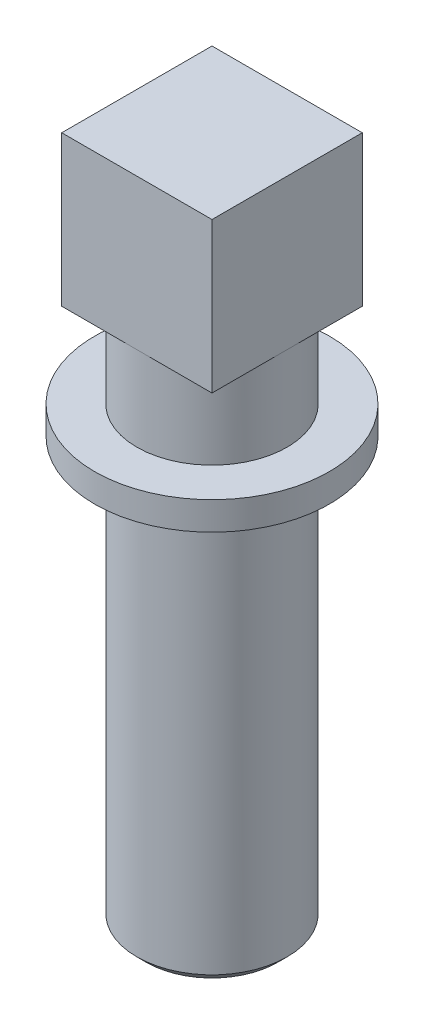
SolidWorks part; units mm, degrees
material "Plain Carbon Steel"
ref_plane "Front Plane" through (0, 0, 0) normal (0, 0, 1) x (1, 0, 0)
ref_plane "Top Plane" through (0, 0, 0) normal (0, 1, 0) x (1, 0, 0)
ref_plane "Right Plane" through (0, 0, 0) normal (1, 0, 0) x (0, 0, -1)
sketch "Shank Sketch Ø16" plane through (0, 0, 0) normal (0, 1, 0) x (1, 0, 0)
  circle A0 centre (0, 0) radius 8
  dimension "D1" = 16
extrude "Shank Ø16x45" add sketch "Shank Sketch Ø16" along normal blind 45
chamfer "Shank Chamfer 1x45°" distance 1 angle 45 1 edges at (0, 0, 8)
sketch "Collar Sketch Ø25" plane through (0, 45, 0) normal (0, 1, 0) x (1, 0, 0)
  circle A0 centre (0, 0) radius 12.5
  dimension "D1" = 25
extrude "Collar Ø25x3" add sketch "Collar Sketch Ø25" along normal blind 3
sketch "Neck Sketch Ø16" plane through (0, 48, 0) normal (0, 1, 0) x (1, 0, 0)
  circle A0 centre (0, 0) radius 8
  dimension "D1" = 16
extrude "Neck Ø16x9" add sketch "Neck Sketch Ø16" along normal blind 9
sketch "Square Head Sketch 16x16" plane through (0, 57, 0) normal (0, 1, 0) x (1, 0, 0)
  line L1 (-8, 8) -> (8, 8)
  line L2 (-8, 8) -> (-8, -8)
  line L3 (-8, -8) -> (8, -8)
  line L4 (8, 8) -> (8, -8)
  line L5 (-8, 8) -> (8, -8) construction
  line L6 (-8, -8) -> (8, 8) construction
  point P0 (0, 0)
  dimension "D1" = 16
  dimension "D2" = 16
extrude "Square Head 16x16x16" add sketch "Square Head Sketch 16x16" along normal blind 16
